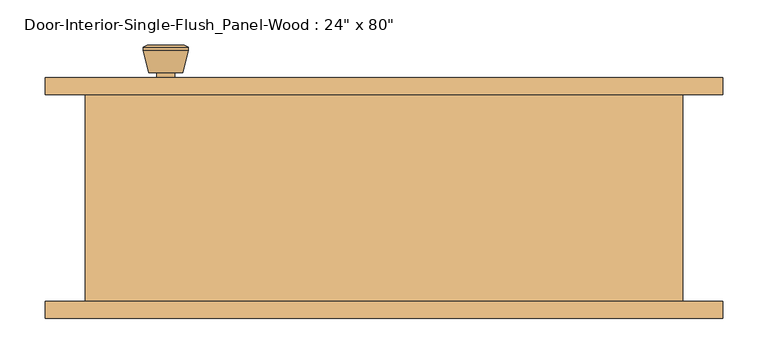
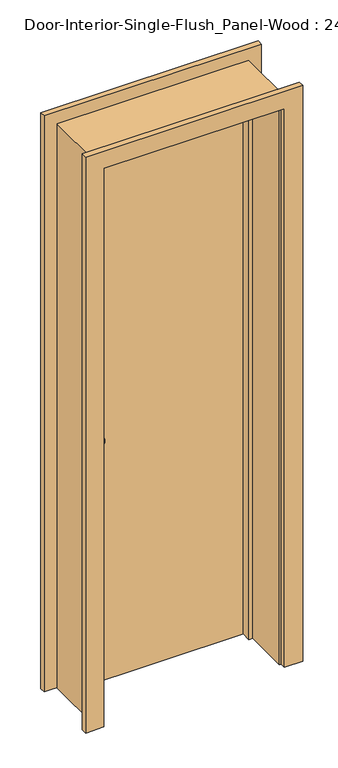
"""IFC4 building model written with IfcOpenShell, lengths in millimetres: door geometry."""

from ifc_helpers import new_model, si_unit, point, frame, frame_2d, origin, origin_with_axes, place, context, project, spatial, polyline, circle_curve, trimmed, segment, composite_curve, outline, extrude, faceted_brep, source, transform, mapped, element, save
from ifc_brep_helpers import plane_surface, cylinder_surface, revolved_surface, advanced_brep


def door_bae2a1e9(model_context):
    return source(origin(), model_context, "Body", "SolidModel", [
        advanced_brep(
        [(-241.3, 70.2, 914.4), (-231.3, 70.2, 914.4), (-251.3, 70.2, 914.4), (-220.8241324, 21.2, 914.4), (-241.3, 21.2, 914.4), (-261.7758676, 21.2, 914.4), (-216.3, 23.0278681, 914.4), (-266.3, 23.0278681, 914.4), (-216.3, 26.4915463, 914.4), (-266.3, 26.4915463, 914.4), (-222.663764, 51.2, 914.4), (-259.936236, 51.2, 914.4), (-231.3, 51.2, 914.4), (-251.3, 51.2, 914.4)],
        [
            (0, 1),
            (1, 2, circle_curve(frame((-241.3, 70.2, 914.4), z_axis=(0.0, 1.0, 0.0), x_axis=(-1.0, 0.0, 0.0)), 10.0)),
            (2, 0),
            (2, 1, circle_curve(frame((-241.3, 70.2, 914.4), z_axis=(0.0, 1.0, 0.0), x_axis=(-1.0, 0.0, 0.0)), 10.0)),
            (3, 4),
            (4, 5),
            (5, 3, circle_curve(frame((-241.3, 21.2, 914.4), z_axis=(0.0, -1.0, 0.0), x_axis=(-1.0, 0.0, 0.0)), 20.4758676)),
            (3, 5, circle_curve(frame((-241.3, 21.2, 914.4), z_axis=(0.0, -1.0, 0.0), x_axis=(-1.0, 0.0, 0.0)), 20.4758676)),
            (6, 3),
            (5, 7),
            (7, 6, circle_curve(frame((-241.3, 23.0278681, 914.4), z_axis=(0.0, -1.0, 0.0), x_axis=(-1.0, 0.0, 0.0)), 25.0)),
            (6, 7, circle_curve(frame((-241.3, 23.0278681, 914.4), z_axis=(0.0, -1.0, 0.0), x_axis=(-1.0, 0.0, 0.0)), 25.0)),
            (8, 6),
            (7, 9),
            (9, 8, circle_curve(frame((-241.3, 26.4915463, 914.4), z_axis=(0.0, -1.0, 0.0), x_axis=(-1.0, 0.0, 0.0)), 25.0)),
            (8, 9, circle_curve(frame((-241.3, 26.4915463, 914.4), z_axis=(0.0, -1.0, 0.0), x_axis=(-1.0, 0.0, 0.0)), 25.0)),
            (10, 8),
            (9, 11),
            (11, 10, circle_curve(frame((-241.3, 51.2, 914.4), z_axis=(0.0, -1.0, 0.0), x_axis=(-1.0, 0.0, 0.0)), 18.636236)),
            (10, 11, circle_curve(frame((-241.3, 51.2, 914.4), z_axis=(0.0, -1.0, 0.0), x_axis=(-1.0, 0.0, 0.0)), 18.636236)),
            (12, 10),
            (11, 13),
            (13, 12, circle_curve(frame((-241.3, 51.2, 914.4), z_axis=(0.0, -1.0, 0.0), x_axis=(-1.0, 0.0, 0.0)), 10.0)),
            (12, 13, circle_curve(frame((-241.3, 51.2, 914.4), z_axis=(0.0, -1.0, 0.0), x_axis=(-1.0, 0.0, 0.0)), 10.0)),
            (1, 12),
            (13, 2),
        ],
        [
            plane_surface(frame((-241.3, 70.2, 914.4), z_axis=(0.0, 1.0, 0.0), x_axis=(-1.0, 0.0, 0.0))),
            plane_surface(frame((-241.3, 21.2, 914.4), z_axis=(0.0, -1.0, 0.0), x_axis=(-1.0, 0.0, 0.0))),
            revolved_surface(polyline([(-261.7758676, 21.2, 914.4), (-266.3, 23.0278681, 914.4)]), (-241.3, 70.2, 914.4), (0.0, 1.0, 0.0)),
            cylinder_surface(frame((-241.3, 70.2, 914.4), z_axis=(0.0, 1.0, 0.0), x_axis=(-1.0, 0.0, 0.0)), 25.0),
            revolved_surface(polyline([(-266.3, 26.4915463, 914.4), (-259.936236, 51.2, 914.4)]), (-241.3, 70.2, 914.4), (0.0, 1.0, 0.0)),
            plane_surface(frame((-241.3, 51.2, 914.4), z_axis=(0.0, 1.0, 0.0), x_axis=(-1.0, 0.0, 0.0))),
            cylinder_surface(frame((-241.3, 70.2, 914.4), z_axis=(0.0, 1.0, 0.0), x_axis=(-1.0, 0.0, 0.0)), 10.0),
        ],
        [
            (0, [[1, 2, 3]]),
            (0, [[-3, 4, -1]]),
            (1, [[5, 6, 7]]),
            (1, [[-6, -5, 8]]),
            (2, [[9, -7, 10, 11]]),
            (2, [[-10, -8, -9, 12]]),
            (3, [[13, -11, 14, 15]]),
            (3, [[-14, -12, -13, 16]]),
            (4, [[17, -15, 18, 19]]),
            (4, [[-18, -16, -17, 20]]),
            (5, [[21, -19, 22, 23]]),
            (5, [[-22, -20, -21, 24]]),
            (6, [[25, -23, 26, -2]]),
            (6, [[-26, -24, -25, -4]]),
        ],
    ),
        extrude(outline(composite_curve([segment(trimmed(circle_curve(frame_2d((914.4, -241.3)), 30.0), [point((914.4, -271.3))], [point((914.4, -211.3))], False, "CARTESIAN"), True, "CONTINUOUS"), segment(trimmed(circle_curve(frame_2d((914.4, -241.3)), 30.0), [point((914.4, -211.3))], [point((914.4, -271.3))], False, "CARTESIAN"), True, "CONTINUOUS")], self_intersect=False)), frame((0.0, 70.2, 0.0), z_axis=(0.0, 1.0, 0.0), x_axis=(0.0, 0.0, 1.0)), (0.0, 0.0, 1.0), 6.0),
        advanced_brep(
        [(-241.3, 117.125, 914.4), (-251.3, 117.125, 914.4), (-231.3, 117.125, 914.4), (-220.8241324, 166.125, 914.4), (-261.7758676, 166.125, 914.4), (-241.3, 166.125, 914.4), (-216.3, 164.2971319, 914.4), (-266.3, 164.2971319, 914.4), (-216.3, 160.8334537, 914.4), (-266.3, 160.8334537, 914.4), (-222.663764, 136.125, 914.4), (-259.936236, 136.125, 914.4), (-231.3, 136.125, 914.4), (-251.3, 136.125, 914.4)],
        [
            (0, 1),
            (1, 2, circle_curve(frame((-241.3, 117.125, 914.4), z_axis=(0.0, -1.0, 0.0), x_axis=(-1.0, 0.0, 0.0)), 10.0)),
            (2, 0),
            (2, 1, circle_curve(frame((-241.3, 117.125, 914.4), z_axis=(0.0, -1.0, 0.0), x_axis=(-1.0, 0.0, 0.0)), 10.0)),
            (3, 4, circle_curve(frame((-241.3, 166.125, 914.4), z_axis=(0.0, 1.0, 0.0), x_axis=(-1.0, 0.0, 0.0)), 20.4758676)),
            (4, 5),
            (5, 3),
            (4, 3, circle_curve(frame((-241.3, 166.125, 914.4), z_axis=(0.0, 1.0, 0.0), x_axis=(-1.0, 0.0, 0.0)), 20.4758676)),
            (6, 7, circle_curve(frame((-241.3, 164.2971319, 914.4), z_axis=(0.0, 1.0, 0.0), x_axis=(-1.0, 0.0, 0.0)), 25.0)),
            (7, 4),
            (3, 6),
            (7, 6, circle_curve(frame((-241.3, 164.2971319, 914.4), z_axis=(0.0, 1.0, 0.0), x_axis=(-1.0, 0.0, 0.0)), 25.0)),
            (8, 9, circle_curve(frame((-241.3, 160.8334537, 914.4), z_axis=(0.0, 1.0, 0.0), x_axis=(-1.0, 0.0, 0.0)), 25.0)),
            (9, 7),
            (6, 8),
            (9, 8, circle_curve(frame((-241.3, 160.8334537, 914.4), z_axis=(0.0, 1.0, 0.0), x_axis=(-1.0, 0.0, 0.0)), 25.0)),
            (10, 11, circle_curve(frame((-241.3, 136.125, 914.4), z_axis=(0.0, 1.0, 0.0), x_axis=(-1.0, 0.0, 0.0)), 18.636236)),
            (11, 9),
            (8, 10),
            (11, 10, circle_curve(frame((-241.3, 136.125, 914.4), z_axis=(0.0, 1.0, 0.0), x_axis=(-1.0, 0.0, 0.0)), 18.636236)),
            (12, 13, circle_curve(frame((-241.3, 136.125, 914.4), z_axis=(0.0, 1.0, 0.0), x_axis=(-1.0, 0.0, 0.0)), 10.0)),
            (13, 11),
            (10, 12),
            (13, 12, circle_curve(frame((-241.3, 136.125, 914.4), z_axis=(0.0, 1.0, 0.0), x_axis=(-1.0, 0.0, 0.0)), 10.0)),
            (1, 13),
            (12, 2),
        ],
        [
            plane_surface(frame((-241.3, 117.125, 914.4), z_axis=(0.0, -1.0, 0.0), x_axis=(-1.0, 0.0, 0.0))),
            plane_surface(frame((-241.3, 166.125, 914.4), z_axis=(0.0, 1.0, 0.0), x_axis=(-1.0, 0.0, 0.0))),
            revolved_surface(polyline([(-261.7758676, 166.125, 914.4), (-266.3, 164.2971319, 914.4)]), (-241.3, 117.125, 914.4), (0.0, -1.0, 0.0)),
            cylinder_surface(frame((-241.3, 117.125, 914.4), z_axis=(0.0, -1.0, 0.0), x_axis=(-1.0, 0.0, 0.0)), 25.0),
            revolved_surface(polyline([(-266.3, 160.8334537, 914.4), (-259.936236, 136.125, 914.4)]), (-241.3, 117.125, 914.4), (0.0, -1.0, 0.0)),
            plane_surface(frame((-241.3, 136.125, 914.4), z_axis=(0.0, -1.0, 0.0), x_axis=(-1.0, 0.0, 0.0))),
            cylinder_surface(frame((-241.3, 117.125, 914.4), z_axis=(0.0, -1.0, 0.0), x_axis=(-1.0, 0.0, 0.0)), 10.0),
        ],
        [
            (0, [[1, 2, 3]]),
            (0, [[-3, 4, -1]]),
            (1, [[5, 6, 7]]),
            (1, [[8, -7, -6]]),
            (2, [[9, 10, -5, 11]]),
            (2, [[12, -11, -8, -10]]),
            (3, [[13, 14, -9, 15]]),
            (3, [[16, -15, -12, -14]]),
            (4, [[17, 18, -13, 19]]),
            (4, [[20, -19, -16, -18]]),
            (5, [[21, 22, -17, 23]]),
            (5, [[24, -23, -20, -22]]),
            (6, [[-2, 25, -21, 26]]),
            (6, [[-4, -26, -24, -25]]),
        ],
    ),
        extrude(outline(composite_curve([segment(trimmed(circle_curve(frame_2d((914.4, -241.3)), 30.0), [point((914.4, -271.3))], [point((914.4, -211.3))], False, "CARTESIAN"), True, "CONTINUOUS"), segment(trimmed(circle_curve(frame_2d((914.4, -241.3)), 30.0), [point((914.4, -211.3))], [point((914.4, -271.3))], False, "CARTESIAN"), True, "CONTINUOUS")], self_intersect=False)), frame((0.0, 111.125, 0.0), z_axis=(0.0, 1.0, 0.0), x_axis=(0.0, 0.0, 1.0)), (0.0, 0.0, 1.0), 6.0),
        faceted_brep([(330.2, 111.125, 0.0), (330.2, -117.475, 0.0), (304.8, -117.475, 0.0), (304.8, 41.275, 0.0), (292.1, 41.275, 0.0), (292.1, 76.2, 0.0), (304.8, 76.2, 0.0), (304.8, 111.125, 0.0), (330.2, 111.125, 2057.4), (330.2, -117.475, 2057.4), (-330.2, -117.475, 2057.4), (-330.2, -117.475, 0.0), (-304.8, -117.475, 0.0), (-304.8, -117.475, 2032.0), (304.8, -117.475, 2032.0), (304.8, 41.275, 2032.0), (-304.8, 41.275, 2032.0), (-304.8, 41.275, 0.0), (-292.1, 41.275, 0.0), (-292.1, 41.275, 2019.3), (292.1, 41.275, 2019.3), (292.1, 76.2, 2019.3), (-292.1, 76.2, 2019.3), (-292.1, 76.2, 0.0), (-304.8, 76.2, 0.0), (-304.8, 76.2, 2032.0), (304.8, 76.2, 2032.0), (304.8, 111.125, 2032.0), (-304.8, 111.125, 2032.0), (-304.8, 111.125, 0.0), (-330.2, 111.125, 0.0), (-330.2, 111.125, 2057.4)], [[[0, 1, 2, 3, 4, 5, 6, 7]], [[1, 0, 8, 9]], [[2, 1, 9, 10, 11, 12, 13, 14]], [[3, 2, 14, 15]], [[4, 3, 15, 16, 17, 18, 19, 20]], [[5, 4, 20, 21]], [[6, 5, 21, 22, 23, 24, 25, 26]], [[7, 6, 26, 27]], [[0, 7, 27, 28, 29, 30, 31, 8]], [[9, 8, 31, 10]], [[15, 14, 13, 16]], [[21, 20, 19, 22]], [[27, 26, 25, 28]], [[30, 29, 24, 23, 18, 17, 12, 11]], [[10, 31, 30, 11]], [[16, 13, 12, 17]], [[22, 19, 18, 23]], [[28, 25, 24, 29]]]),
        extrude(outline(polyline([(304.8, 76.2), (-304.8, 76.2), (-304.8, 111.125), (304.8, 111.125), (304.8, 76.2)])), origin_with_axes(), (0.0, 0.0, 1.0), 2032.0),
        extrude(outline(polyline([(0.0, 311.15), (0.0, 374.65), (2101.85, 374.65), (2101.85, -374.65), (0.0, -374.65), (0.0, -311.15), (2038.35, -311.15), (2038.35, 311.15), (0.0, 311.15)])), frame((0.0, 111.125, 0.0), z_axis=(0.0, 1.0, 0.0), x_axis=(0.0, 0.0, 1.0)), (0.0, 0.0, 1.0), 19.05),
        extrude(outline(polyline([(0.0, 311.15), (0.0, 374.65), (2101.85, 374.65), (2101.85, -374.65), (0.0, -374.65), (0.0, -311.15), (2038.35, -311.15), (2038.35, 311.15), (0.0, 311.15)])), frame((0.0, -136.525, 0.0), z_axis=(0.0, 1.0, 0.0), x_axis=(0.0, 0.0, 1.0)), (0.0, 0.0, 1.0), 19.05),
    ])


if __name__ == "__main__":
    model = new_model("IFC4")
    model_context = context("Model", 3, world=origin())
    ifc_project = project(units=[si_unit("LENGTHUNIT", "METRE", prefix="MILLI")], contexts=[model_context])
    site = spatial("IfcSite", under=ifc_project)
    building = spatial("IfcBuilding", under=site)
    placement = place(None, origin())
    door_shape = door_bae2a1e9(model_context)
    element("IfcDoor", 1, ObjectType="Door-Interior-Single-Flush_Panel-Wood : 24\" x 80\"", at=placement, inside=building, context=model_context, shape_type="MappedRepresentation", body=[
        mapped(door_shape, transform((0.0, 0.0, 0.0), x_axis=(1.0, 0.0, 0.0), y_axis=(0.0, 1.0, 0.0), z_axis=(0.0, 0.0, 1.0))),
    ])
    save(model, "model.ifc")

# Revit data of these elements
# Type "Door-Interior-Single-Flush_Panel-Wood : 24\" x 80\""
#   Type Mark = "12"
#   Assembly Code = "C1020300"
#   Analytic Construction = "Wooden"
#   Thickness = 0' - 1 3/8"
#   Thermal Resistance (R) = 2.5876 (h·ft²·°F)/BTU
#   Swing Angle [instance default] = 90.00°
#   Rough Width = 2' - 2"
#   Rough Height = 6' - 9"
#   Height = 6' - 8"
#   Width = 2' - 0"
#   Heat Transfer Coefficient (U) = 0.3865 BTU/(h·ft²·°F)
#   Trim Material = Cherry
#   Panel Material = Cherry
#   Frame Material = Cherry
#   Door Handle Material = Aluminum
#   Visual Light Transmittance = 0
#   Solar Heat Gain Coefficient = 0
#   Wall Closure = (empty or 0)
#   Function = (empty or 0)
# Element 1 (IfcDoor, "Door-Interior-Single-Flush_Panel-Wood : 24\" x 80\"")
#   Materials on its faces: "Cherry", "Aluminum"
# Materials
#   "Cherry": class "Wood", colour RGB 226 177 128, transparency 0, Description = "Prunus Serotina", Cost = 0
#   "Aluminum": class "Metal", colour RGB 247 247 247, transparency 0, Description = "Aluminum 6061", Cost = 0
